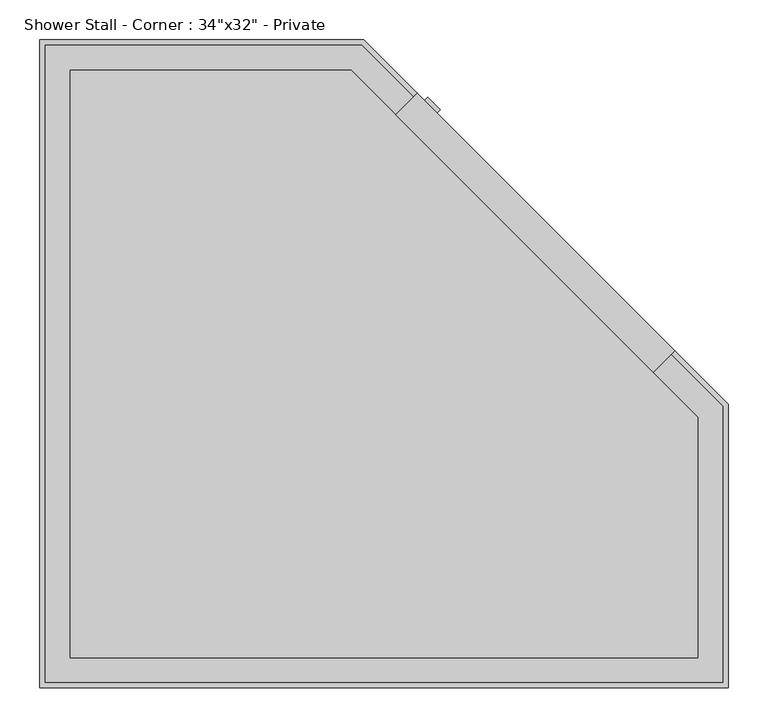
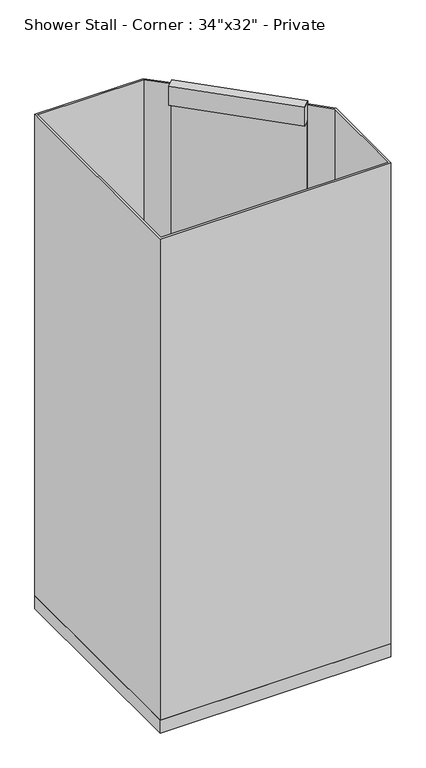
"""IFC4 building model written with IfcOpenShell, lengths in millimetres: flow terminal geometry."""

from ifc_helpers import new_model, si_unit, point, frame, frame_2d, origin, origin_with_axes, place, context, project, spatial, polyline, circle_curve, trimmed, segment, composite_curve, outline, extrude, faceted_brep, source, transform, mapped, element, save


def flow_terminal_2596653b(model_context):
    return source(origin(), model_context, "Body", "SolidModel", [
        faceted_brep([(0.0, 0.0, 50.8), (863.6, 0.0, 50.8), (863.6, 355.6, 50.8), (406.4, 812.8, 50.8), (0.0, 812.8, 50.8), (825.5, 38.1, 50.8), (38.1, 38.1, 50.8), (38.1, 774.7, 50.8), (390.6184633, 774.7, 50.8), (825.5, 339.8184633, 50.8), (0.0, 0.0, 0.0), (0.0, 812.8, 0.0), (406.4, 812.8, 0.0), (863.6, 355.6, 0.0), (863.6, 0.0, 0.0), (38.1, 38.1, 38.1), (825.5, 38.1, 38.1), (825.5, 339.8184633, 38.1), (390.6184633, 774.7, 38.1), (38.1, 774.7, 38.1)], [[[0, 1, 2, 3, 4], [5, 6, 7, 8, 9]], [[10, 11, 12, 13, 14]], [[1, 0, 10, 14]], [[2, 1, 14, 13]], [[3, 2, 13, 12]], [[4, 3, 12, 11]], [[0, 4, 11, 10]], [[15, 16, 17, 18, 19]], [[16, 15, 6, 5]], [[17, 16, 5, 9]], [[18, 17, 9, 8]], [[19, 18, 8, 7]], [[15, 19, 7, 6]]]),
        extrude(outline(composite_curve([segment(trimmed(circle_curve(frame_2d((431.8, 406.4)), 31.75), [point((400.05, 406.4))], [point((463.55, 406.4))], False, "CARTESIAN"), True, "CONTINUOUS"), segment(trimmed(circle_curve(frame_2d((431.8, 406.4)), 31.75), [point((463.55, 406.4))], [point((400.05, 406.4))], False, "CARTESIAN"), True, "CONTINUOUS")], self_intersect=False)), origin_with_axes(), (0.0, 0.0, 1.0), 38.1),
        extrude(outline(polyline([(468.8652618, 741.3544821), (473.3553898, 745.8446102), (796.6446102, 422.5553898), (792.1544821, 418.0652618), (468.8652618, 741.3544821)])), frame((0.0, 0.0, 50.8), z_axis=(0.0, 0.0, 1.0), x_axis=(1.0, 0.0, 0.0)), (0.0, 0.0, 1.0), 1841.5),
        extrude(outline(polyline([(473.3553898, 745.8446102), (796.6446102, 422.5553898), (769.7038418, 395.6146215), (446.4146215, 718.9038418), (473.3553898, 745.8446102)])), frame((0.0, 0.0, 1892.3), z_axis=(0.0, 0.0, 1.0), x_axis=(1.0, 0.0, 0.0)), (0.0, 0.0, 1.0), 76.2),
        extrude(outline(polyline([(486.4804954, 741.0092035), (502.1959436, 725.2937553), (498.0510942, 721.1489058), (482.3356459, 736.8643541), (486.4804954, 741.0092035)])), frame((0.0, 0.0, 882.65), z_axis=(0.0, 0.0, 1.0), x_axis=(1.0, 0.0, 0.0)), (0.0, 0.0, 1.0), 107.95),
        extrude(outline(polyline([(406.4, 812.8), (473.3553898, 745.8446102), (468.8652618, 741.3544821), (403.7697439, 806.45), (6.35, 806.45), (6.35, 6.35), (857.25, 6.35), (857.25, 352.9697439), (792.1544821, 418.0652618), (796.6446102, 422.5553898), (863.6, 355.6), (863.6, 0.0), (0.0, 0.0), (0.0, 812.8), (406.4, 812.8)])), frame((0.0, 0.0, 50.8), z_axis=(0.0, 0.0, 1.0), x_axis=(1.0, 0.0, 0.0)), (0.0, 0.0, 1.0), 1905.0),
    ])


if __name__ == "__main__":
    model = new_model("IFC4")
    model_context = context("Model", 3, world=origin())
    ifc_project = project(units=[si_unit("LENGTHUNIT", "METRE", prefix="MILLI")], contexts=[model_context])
    site = spatial("IfcSite", under=ifc_project)
    building = spatial("IfcBuilding", under=site)
    placement = place(None, origin())
    flow_terminal_shape = flow_terminal_2596653b(model_context)
    element("IfcFlowTerminal", 1, ObjectType="Shower Stall - Corner : 34\"x32\" - Private", at=placement, inside=building, context=model_context, shape_type="MappedRepresentation", body=[
        mapped(flow_terminal_shape, transform((0.0, 0.0, 0.0), x_axis=(1.0, 0.0, 0.0), y_axis=(0.0, 1.0, 0.0), z_axis=(0.0, 0.0, 1.0))),
    ])
    save(model, "model.ifc")

# Revit data of these elements
# Type "Shower Stall - Corner : 34\"x32\" - Private"
#   Width 1 = 0' - 0.88388"
#   WFU = 2
#   Shower Width = 2' - 8"
#   Shower Length = 2' - 10"
#   Shower Height = 6' - 5"
#   Sanitary Radius = 1"
#   Sanitary Diameter = 2"
#   Length 1 = 1' - 4"
#   Hot Water Radius = 1/4"
#   Hot Water Diameter = 1/2"
#   Height 1 = 3' - 3"
#   Half Door Width = 0' - 9"
#   HWFU = 1
#   Flow Pressure [instance default] = 8.00 psi
#   Door Width = 1' - 6"
#   Cold Water Radius = 1/4"
#   Cold Water Diameter = 1/2"
#   CWFU = 1
#   Shower Stall Material = none
#   Door Material = none
#   Door Handle Material = none
#   Default Elevation = 0
